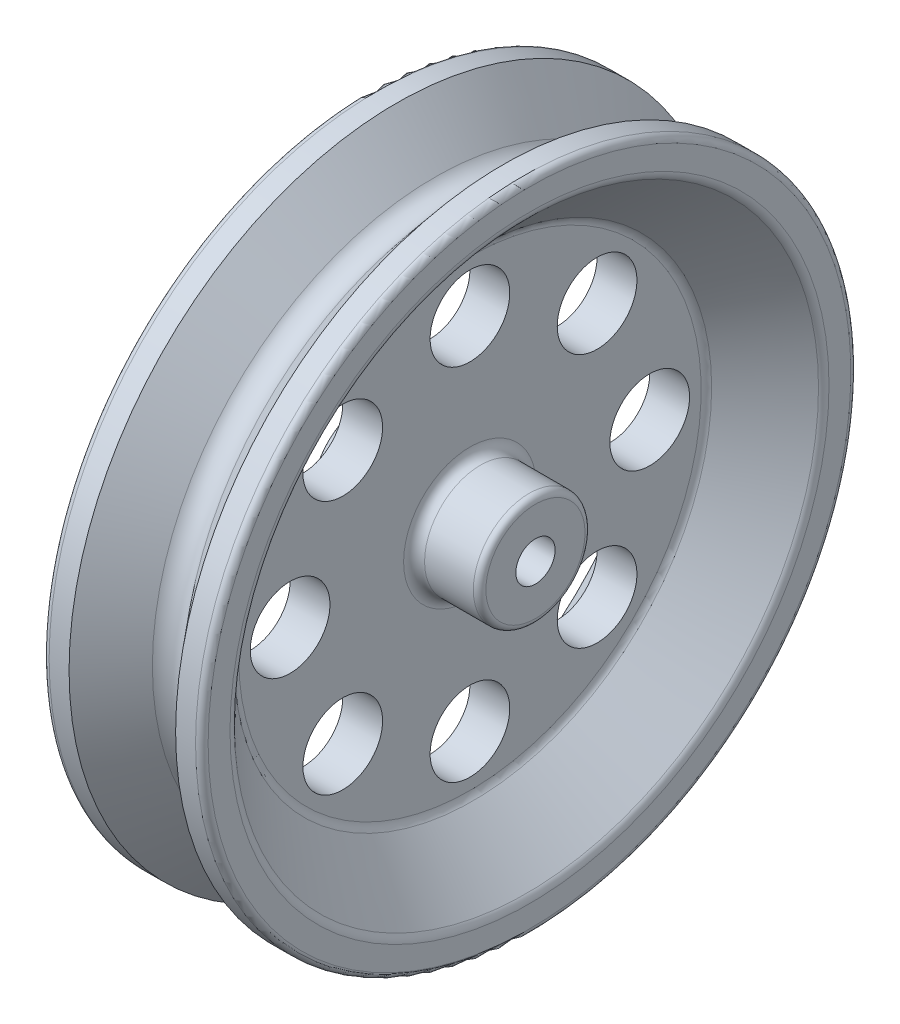
ISO-10303-21;
HEADER;
FILE_DESCRIPTION(('STEP AP214'),'2;1');
FILE_NAME('part.step','',(''),(''),'','','');
FILE_SCHEMA(('AUTOMOTIVE_DESIGN { 1 0 10303 214 1 1 1 1 }'));
ENDSEC;
DATA;
#1=APPLICATION_CONTEXT('core data for automotive mechanical design processes');
#2=APPLICATION_PROTOCOL_DEFINITION('international standard','automotive_design',2000,#1);
#3=PRODUCT_CONTEXT('',#1,'mechanical');
#4=PRODUCT('Part','Part','',(#3));
#5=PRODUCT_RELATED_PRODUCT_CATEGORY('part','',(#4));
#6=PRODUCT_DEFINITION_FORMATION('','',#4);
#7=PRODUCT_DEFINITION_CONTEXT('part definition',#1,'design');
#8=PRODUCT_DEFINITION('design','',#6,#7);
#9=PRODUCT_DEFINITION_SHAPE('','',#8);
#10=(LENGTH_UNIT() NAMED_UNIT(*) SI_UNIT(.MILLI.,.METRE.));
#11=(NAMED_UNIT(*) PLANE_ANGLE_UNIT() SI_UNIT($,.RADIAN.));
#12=(NAMED_UNIT(*) SI_UNIT($,.STERADIAN.) SOLID_ANGLE_UNIT());
#13=UNCERTAINTY_MEASURE_WITH_UNIT(LENGTH_MEASURE(1.E-05),#10,'distance_accuracy_value','');
#14=(GEOMETRIC_REPRESENTATION_CONTEXT(3) GLOBAL_UNCERTAINTY_ASSIGNED_CONTEXT((#13)) GLOBAL_UNIT_ASSIGNED_CONTEXT((#10,
#11,#12)) REPRESENTATION_CONTEXT('',''));
#15=CARTESIAN_POINT('',(0.,0.,0.));
#16=DIRECTION('',(0.,0.,1.));
#17=DIRECTION('',(1.,0.,0.));
#18=AXIS2_PLACEMENT_3D('',#15,#16,#17);
#19=CARTESIAN_POINT('',(0.,0.,0.));
#20=DIRECTION('',(-1.,0.,0.));
#21=DIRECTION('',(0.,0.,1.));
#22=AXIS2_PLACEMENT_3D('',#19,#20,#21);
#23=CYLINDRICAL_SURFACE('',#22,0.5325);
#24=CARTESIAN_POINT('',(-0.755,0.,0.));
#25=DIRECTION('',(1.,0.,0.));
#26=DIRECTION('',(0.,0.,-1.));
#27=AXIS2_PLACEMENT_3D('',#24,#25,#26);
#28=CIRCLE('',#27,0.5325);
#29=CARTESIAN_POINT('',(-0.755,0.,-0.5325));
#30=VERTEX_POINT('',#29);
#31=EDGE_CURVE('E10',#30,#30,#28,.T.);
#32=ORIENTED_EDGE('',*,*,#31,.T.);
#33=EDGE_LOOP('',(#32));
#34=FACE_BOUND('',#33,.T.);
#35=CARTESIAN_POINT('',(-0.29,0.,0.));
#36=DIRECTION('',(1.,0.,0.));
#37=DIRECTION('',(0.,0.,-1.));
#38=AXIS2_PLACEMENT_3D('',#35,#36,#37);
#39=CIRCLE('',#38,0.5325);
#40=CARTESIAN_POINT('',(-0.29,0.,-0.5325));
#41=VERTEX_POINT('',#40);
#42=EDGE_CURVE('E83',#41,#41,#39,.F.);
#43=ORIENTED_EDGE('',*,*,#42,.T.);
#44=EDGE_LOOP('',(#43));
#45=FACE_BOUND('',#44,.T.);
#46=ADVANCED_FACE('F40',(#34,#45),#23,.T.);
#47=CARTESIAN_POINT('',(-0.815,0.1875,0.));
#48=DIRECTION('',(1.,0.,0.));
#49=DIRECTION('',(0.,0.,-1.));
#50=AXIS2_PLACEMENT_3D('',#47,#48,#49);
#51=PLANE('',#50);
#52=CARTESIAN_POINT('',(-0.815,0.,0.));
#53=DIRECTION('',(1.,0.,0.));
#54=DIRECTION('',(0.,0.,-1.));
#55=AXIS2_PLACEMENT_3D('',#52,#53,#54);
#56=CIRCLE('',#55,0.4725);
#57=CARTESIAN_POINT('',(-0.815,0.,-0.4725));
#58=VERTEX_POINT('',#57);
#59=EDGE_CURVE('E42',#58,#58,#56,.F.);
#60=ORIENTED_EDGE('',*,*,#59,.T.);
#61=EDGE_LOOP('',(#60));
#62=FACE_BOUND('',#61,.T.);
#63=CARTESIAN_POINT('',(-0.815,0.,0.));
#64=DIRECTION('',(-1.,0.,0.));
#65=DIRECTION('',(0.,0.,1.));
#66=AXIS2_PLACEMENT_3D('',#63,#64,#65);
#67=CIRCLE('',#66,0.1875);
#68=CARTESIAN_POINT('',(-0.815,0.,0.1875));
#69=VERTEX_POINT('',#68);
#70=EDGE_CURVE('E104',#69,#69,#67,.T.);
#71=ORIENTED_EDGE('',*,*,#70,.F.);
#72=EDGE_LOOP('',(#71));
#73=FACE_BOUND('',#72,.T.);
#74=ADVANCED_FACE('F208',(#62,#73),#51,.F.);
#75=CARTESIAN_POINT('',(0.,0.,0.));
#76=DIRECTION('',(-1.,0.,0.));
#77=DIRECTION('',(0.,0.,1.));
#78=AXIS2_PLACEMENT_3D('',#75,#76,#77);
#79=CYLINDRICAL_SURFACE('',#78,0.1875);
#80=CARTESIAN_POINT('',(0.815,0.,0.));
#81=DIRECTION('',(-1.,0.,0.));
#82=DIRECTION('',(0.,0.,1.));
#83=AXIS2_PLACEMENT_3D('',#80,#81,#82);
#84=CIRCLE('',#83,0.1875);
#85=CARTESIAN_POINT('',(0.815,0.,0.1875));
#86=VERTEX_POINT('',#85);
#87=EDGE_CURVE('E107',#86,#86,#84,.T.);
#88=ORIENTED_EDGE('',*,*,#87,.F.);
#89=EDGE_LOOP('',(#88));
#90=FACE_BOUND('',#89,.T.);
#91=ORIENTED_EDGE('',*,*,#70,.T.);
#92=EDGE_LOOP('',(#91));
#93=FACE_BOUND('',#92,.T.);
#94=ADVANCED_FACE('F213',(#90,#93),#79,.F.);
#95=CARTESIAN_POINT('',(0.815,0.1875,0.));
#96=DIRECTION('',(-1.,0.,0.));
#97=DIRECTION('',(0.,0.,1.));
#98=AXIS2_PLACEMENT_3D('',#95,#96,#97);
#99=PLANE('',#98);
#100=CARTESIAN_POINT('',(0.815,0.,0.));
#101=DIRECTION('',(-1.,0.,0.));
#102=DIRECTION('',(0.,0.,1.));
#103=AXIS2_PLACEMENT_3D('',#100,#101,#102);
#104=CIRCLE('',#103,0.4725);
#105=CARTESIAN_POINT('',(0.815,0.,0.4725));
#106=VERTEX_POINT('',#105);
#107=EDGE_CURVE('E48',#106,#106,#104,.F.);
#108=ORIENTED_EDGE('',*,*,#107,.T.);
#109=EDGE_LOOP('',(#108));
#110=FACE_BOUND('',#109,.T.);
#111=ORIENTED_EDGE('',*,*,#87,.T.);
#112=EDGE_LOOP('',(#111));
#113=FACE_BOUND('',#112,.T.);
#114=ADVANCED_FACE('F282',(#110,#113),#99,.F.);
#115=CARTESIAN_POINT('',(0.,0.,0.));
#116=DIRECTION('',(-1.,0.,0.));
#117=DIRECTION('',(0.,0.,1.));
#118=AXIS2_PLACEMENT_3D('',#115,#116,#117);
#119=CYLINDRICAL_SURFACE('',#118,0.5325);
#120=CARTESIAN_POINT('',(0.755,0.,0.));
#121=DIRECTION('',(-1.,0.,0.));
#122=DIRECTION('',(0.,0.,1.));
#123=AXIS2_PLACEMENT_3D('',#120,#121,#122);
#124=CIRCLE('',#123,0.5325);
#125=CARTESIAN_POINT('',(0.755,0.,0.5325));
#126=VERTEX_POINT('',#125);
#127=EDGE_CURVE('E55',#126,#126,#124,.T.);
#128=ORIENTED_EDGE('',*,*,#127,.T.);
#129=EDGE_LOOP('',(#128));
#130=FACE_BOUND('',#129,.T.);
#131=CARTESIAN_POINT('',(0.29,0.,0.));
#132=DIRECTION('',(-1.,0.,0.));
#133=DIRECTION('',(0.,0.,1.));
#134=AXIS2_PLACEMENT_3D('',#131,#132,#133);
#135=CIRCLE('',#134,0.5325);
#136=CARTESIAN_POINT('',(0.29,0.,0.5325));
#137=VERTEX_POINT('',#136);
#138=EDGE_CURVE('E82',#137,#137,#135,.F.);
#139=ORIENTED_EDGE('',*,*,#138,.T.);
#140=EDGE_LOOP('',(#139));
#141=FACE_BOUND('',#140,.T.);
#142=ADVANCED_FACE('F283',(#130,#141),#119,.T.);
#143=CARTESIAN_POINT('',(0.19,0.5325,0.));
#144=DIRECTION('',(-1.,0.,0.));
#145=DIRECTION('',(0.,0.,1.));
#146=AXIS2_PLACEMENT_3D('',#143,#144,#145);
#147=PLANE('',#146);
#148=CARTESIAN_POINT('',(0.19,0.,-1.715));
#149=DIRECTION('',(-1.,0.,0.));
#150=DIRECTION('',(0.,0.,1.));
#151=AXIS2_PLACEMENT_3D('',#148,#149,#150);
#152=CIRCLE('',#151,0.38);
#153=CARTESIAN_POINT('',(0.19,0.,-1.335));
#154=VERTEX_POINT('',#153);
#155=EDGE_CURVE('E129',#154,#154,#152,.T.);
#156=ORIENTED_EDGE('',*,*,#155,.T.);
#157=EDGE_LOOP('',(#156));
#158=FACE_BOUND('',#157,.T.);
#159=CARTESIAN_POINT('',(0.19,-1.21268812973494,-1.21268812973492));
#160=DIRECTION('',(-1.,0.,0.));
#161=DIRECTION('',(0.,0.,1.));
#162=AXIS2_PLACEMENT_3D('',#159,#160,#161);
#163=CIRCLE('',#162,0.38);
#164=CARTESIAN_POINT('',(0.19,-1.21268812973494,-0.832688129734923));
#165=VERTEX_POINT('',#164);
#166=EDGE_CURVE('E135',#165,#165,#163,.T.);
#167=ORIENTED_EDGE('',*,*,#166,.T.);
#168=EDGE_LOOP('',(#167));
#169=FACE_BOUND('',#168,.T.);
#170=CARTESIAN_POINT('',(0.19,-1.715,0.));
#171=DIRECTION('',(-1.,0.,0.));
#172=DIRECTION('',(0.,0.,1.));
#173=AXIS2_PLACEMENT_3D('',#170,#171,#172);
#174=CIRCLE('',#173,0.38);
#175=CARTESIAN_POINT('',(0.19,-1.715,0.38));
#176=VERTEX_POINT('',#175);
#177=EDGE_CURVE('E132',#176,#176,#174,.T.);
#178=ORIENTED_EDGE('',*,*,#177,.T.);
#179=EDGE_LOOP('',(#178));
#180=FACE_BOUND('',#179,.T.);
#181=CARTESIAN_POINT('',(0.19,-1.21268812973492,1.21268812973494));
#182=DIRECTION('',(-1.,0.,0.));
#183=DIRECTION('',(0.,0.,1.));
#184=AXIS2_PLACEMENT_3D('',#181,#182,#183);
#185=CIRCLE('',#184,0.38);
#186=CARTESIAN_POINT('',(0.19,-1.21268812973492,1.59268812973494));
#187=VERTEX_POINT('',#186);
#188=EDGE_CURVE('E136',#187,#187,#185,.T.);
#189=ORIENTED_EDGE('',*,*,#188,.T.);
#190=EDGE_LOOP('',(#189));
#191=FACE_BOUND('',#190,.T.);
#192=CARTESIAN_POINT('',(0.19,0.,1.715));
#193=DIRECTION('',(-1.,0.,0.));
#194=DIRECTION('',(0.,0.,1.));
#195=AXIS2_PLACEMENT_3D('',#192,#193,#194);
#196=CIRCLE('',#195,0.38);
#197=CARTESIAN_POINT('',(0.19,0.,2.095));
#198=VERTEX_POINT('',#197);
#199=EDGE_CURVE('E143',#198,#198,#196,.T.);
#200=ORIENTED_EDGE('',*,*,#199,.T.);
#201=EDGE_LOOP('',(#200));
#202=FACE_BOUND('',#201,.T.);
#203=CARTESIAN_POINT('',(0.19,1.21268812973494,1.21268812973491));
#204=DIRECTION('',(-1.,0.,0.));
#205=DIRECTION('',(0.,0.,1.));
#206=AXIS2_PLACEMENT_3D('',#203,#204,#205);
#207=CIRCLE('',#206,0.38);
#208=CARTESIAN_POINT('',(0.19,1.21268812973494,1.59268812973491));
#209=VERTEX_POINT('',#208);
#210=EDGE_CURVE('E145',#209,#209,#207,.T.);
#211=ORIENTED_EDGE('',*,*,#210,.T.);
#212=EDGE_LOOP('',(#211));
#213=FACE_BOUND('',#212,.T.);
#214=CARTESIAN_POINT('',(0.19,1.21268812973493,-1.21268812973493));
#215=DIRECTION('',(-1.,0.,0.));
#216=DIRECTION('',(0.,0.,1.));
#217=AXIS2_PLACEMENT_3D('',#214,#215,#216);
#218=CIRCLE('',#217,0.38);
#219=CARTESIAN_POINT('',(0.19,1.21268812973493,-0.832688129734931));
#220=VERTEX_POINT('',#219);
#221=EDGE_CURVE('E150',#220,#220,#218,.T.);
#222=ORIENTED_EDGE('',*,*,#221,.T.);
#223=EDGE_LOOP('',(#222));
#224=FACE_BOUND('',#223,.T.);
#225=CARTESIAN_POINT('',(0.19,1.715,0.));
#226=DIRECTION('',(-1.,0.,0.));
#227=DIRECTION('',(0.,0.,1.));
#228=AXIS2_PLACEMENT_3D('',#225,#226,#227);
#229=CIRCLE('',#228,0.38);
#230=CARTESIAN_POINT('',(0.19,1.715,0.38));
#231=VERTEX_POINT('',#230);
#232=EDGE_CURVE('E121',#231,#231,#229,.T.);
#233=ORIENTED_EDGE('',*,*,#232,.T.);
#234=EDGE_LOOP('',(#233));
#235=FACE_BOUND('',#234,.T.);
#236=CARTESIAN_POINT('',(0.19,0.,0.));
#237=DIRECTION('',(-1.,0.,0.));
#238=DIRECTION('',(0.,0.,1.));
#239=AXIS2_PLACEMENT_3D('',#236,#237,#238);
#240=CIRCLE('',#239,0.6325);
#241=CARTESIAN_POINT('',(0.19,0.,0.6325));
#242=VERTEX_POINT('',#241);
#243=EDGE_CURVE('E87',#242,#242,#240,.T.);
#244=ORIENTED_EDGE('',*,*,#243,.T.);
#245=EDGE_LOOP('',(#244));
#246=FACE_BOUND('',#245,.T.);
#247=CARTESIAN_POINT('',(0.19,0.,0.));
#248=DIRECTION('',(-1.,0.,0.));
#249=DIRECTION('',(0.,0.,1.));
#250=AXIS2_PLACEMENT_3D('',#247,#248,#249);
#251=CIRCLE('',#250,2.20543037312372);
#252=CARTESIAN_POINT('',(0.19,0.,2.20543037312372));
#253=VERTEX_POINT('',#252);
#254=EDGE_CURVE('E89',#253,#253,#251,.F.);
#255=ORIENTED_EDGE('',*,*,#254,.T.);
#256=EDGE_LOOP('',(#255));
#257=FACE_BOUND('',#256,.T.);
#258=ADVANCED_FACE('F280',(#158,#169,#180,#191,#202,#213,#224,#235,#246,#257),#147,.F.);
#259=CARTESIAN_POINT('',(0.19,0.,0.));
#260=DIRECTION('',(1.,0.,0.));
#261=DIRECTION('',(0.,0.,-1.));
#262=AXIS2_PLACEMENT_3D('',#259,#260,#261);
#263=CONICAL_SURFACE('',#262,2.24685172936103,0.785398163397447);
#264=CARTESIAN_POINT('',(0.728858948756745,0.,0.));
#265=DIRECTION('',(-1.,0.,0.));
#266=DIRECTION('',(0.,0.,1.));
#267=AXIS2_PLACEMENT_3D('',#264,#265,#266);
#268=CIRCLE('',#267,2.78571067811777);
#269=CARTESIAN_POINT('',(0.728858948756745,0.,2.78571067811777));
#270=VERTEX_POINT('',#269);
#271=EDGE_CURVE('E60',#270,#270,#268,.F.);
#272=ORIENTED_EDGE('',*,*,#271,.T.);
#273=EDGE_LOOP('',(#272));
#274=FACE_BOUND('',#273,.T.);
#275=CARTESIAN_POINT('',(0.219289321881345,0.,0.));
#276=DIRECTION('',(1.,0.,0.));
#277=DIRECTION('',(0.,0.,-1.));
#278=AXIS2_PLACEMENT_3D('',#275,#276,#277);
#279=CIRCLE('',#278,2.27614105124237);
#280=CARTESIAN_POINT('',(0.219289321881345,0.,-2.27614105124237));
#281=VERTEX_POINT('',#280);
#282=EDGE_CURVE('E58',#281,#281,#279,.F.);
#283=ORIENTED_EDGE('',*,*,#282,.T.);
#284=EDGE_LOOP('',(#283));
#285=FACE_BOUND('',#284,.T.);
#286=ADVANCED_FACE('F247',(#274,#285),#263,.F.);
#287=CARTESIAN_POINT('',(0.75814827063809,2.81499999999912,0.));
#288=DIRECTION('',(-1.,0.,0.));
#289=DIRECTION('',(0.,0.,1.));
#290=AXIS2_PLACEMENT_3D('',#287,#288,#289);
#291=PLANE('',#290);
#292=CARTESIAN_POINT('',(0.75814827063809,0.,0.));
#293=DIRECTION('',(-1.,0.,0.));
#294=DIRECTION('',(0.,0.,1.));
#295=AXIS2_PLACEMENT_3D('',#292,#293,#294);
#296=CIRCLE('',#295,2.85642135623643);
#297=CARTESIAN_POINT('',(0.75814827063809,0.,2.85642135623643));
#298=VERTEX_POINT('',#297);
#299=EDGE_CURVE('E61',#298,#298,#296,.T.);
#300=ORIENTED_EDGE('',*,*,#299,.T.);
#301=EDGE_LOOP('',(#300));
#302=FACE_BOUND('',#301,.T.);
#303=CARTESIAN_POINT('',(0.75814827063809,0.,0.));
#304=DIRECTION('',(-1.,0.,0.));
#305=DIRECTION('',(0.,0.,1.));
#306=AXIS2_PLACEMENT_3D('',#303,#304,#305);
#307=CIRCLE('',#306,3.06499999999912);
#308=CARTESIAN_POINT('',(0.75814827063809,0.,3.06499999999912));
#309=VERTEX_POINT('',#308);
#310=EDGE_CURVE('E91',#309,#309,#307,.F.);
#311=ORIENTED_EDGE('',*,*,#310,.T.);
#312=EDGE_LOOP('',(#311));
#313=FACE_BOUND('',#312,.T.);
#314=ADVANCED_FACE('F242',(#302,#313),#291,.F.);
#315=CARTESIAN_POINT('',(0.,0.,0.));
#316=DIRECTION('',(-1.,0.,0.));
#317=DIRECTION('',(0.,0.,1.));
#318=AXIS2_PLACEMENT_3D('',#315,#316,#317);
#319=CYLINDRICAL_SURFACE('',#318,3.12499999999912);
#320=CARTESIAN_POINT('',(0.69814827063809,0.,0.));
#321=DIRECTION('',(-1.,0.,0.));
#322=DIRECTION('',(0.,0.,1.));
#323=AXIS2_PLACEMENT_3D('',#320,#321,#322);
#324=CIRCLE('',#323,3.12499999999912);
#325=CARTESIAN_POINT('',(0.69814827063809,0.,3.12499999999912));
#326=VERTEX_POINT('',#325);
#327=EDGE_CURVE('E96',#326,#326,#324,.T.);
#328=ORIENTED_EDGE('',*,*,#327,.T.);
#329=EDGE_LOOP('',(#328));
#330=FACE_BOUND('',#329,.T.);
#331=CARTESIAN_POINT('',(0.50814827063809,0.,0.));
#332=DIRECTION('',(-1.,0.,0.));
#333=DIRECTION('',(0.,0.,1.));
#334=AXIS2_PLACEMENT_3D('',#331,#332,#333);
#335=CIRCLE('',#334,3.12499999999912);
#336=CARTESIAN_POINT('',(0.50814827063809,0.,3.12499999999912));
#337=VERTEX_POINT('',#336);
#338=EDGE_CURVE('E112',#337,#337,#335,.T.);
#339=ORIENTED_EDGE('',*,*,#338,.F.);
#340=EDGE_LOOP('',(#339));
#341=FACE_BOUND('',#340,.T.);
#342=ADVANCED_FACE('F246',(#330,#341),#319,.T.);
#343=CARTESIAN_POINT('',(0.50814827063809,0.,0.));
#344=DIRECTION('',(1.,0.,0.));
#345=DIRECTION('',(0.,0.,-1.));
#346=AXIS2_PLACEMENT_3D('',#343,#344,#345);
#347=CONICAL_SURFACE('',#346,3.12499999999912,0.872664625997163);
#348=CARTESIAN_POINT('',(0.145548444192605,0.,0.));
#349=DIRECTION('',(-1.,0.,0.));
#350=DIRECTION('',(0.,0.,1.));
#351=AXIS2_PLACEMENT_3D('',#348,#349,#350);
#352=CIRCLE('',#351,2.69287035415868);
#353=CARTESIAN_POINT('',(0.145548444192605,0.,2.69287035415868));
#354=VERTEX_POINT('',#353);
#355=EDGE_CURVE('E111',#354,#354,#352,.T.);
#356=ORIENTED_EDGE('',*,*,#355,.F.);
#357=EDGE_LOOP('',(#356));
#358=FACE_BOUND('',#357,.T.);
#359=ORIENTED_EDGE('',*,*,#338,.T.);
#360=EDGE_LOOP('',(#359));
#361=FACE_BOUND('',#360,.T.);
#362=ADVANCED_FACE('F260',(#358,#361),#347,.T.);
#363=CARTESIAN_POINT('',(0.,0.,0.));
#364=DIRECTION('',(-1.,0.,0.));
#365=DIRECTION('',(0.,0.,1.));
#366=AXIS2_PLACEMENT_3D('',#363,#364,#365);
#367=TOROIDAL_SURFACE('',#366,2.81499999999912,0.19);
#368=CARTESIAN_POINT('',(-0.145548444192604,0.,0.));
#369=DIRECTION('',(-1.,0.,0.));
#370=DIRECTION('',(0.,0.,1.));
#371=AXIS2_PLACEMENT_3D('',#368,#369,#370);
#372=CIRCLE('',#371,2.69287035415867);
#373=CARTESIAN_POINT('',(-0.145548444192604,0.,2.69287035415867));
#374=VERTEX_POINT('',#373);
#375=EDGE_CURVE('E120',#374,#374,#372,.T.);
#376=ORIENTED_EDGE('',*,*,#375,.F.);
#377=EDGE_LOOP('',(#376));
#378=FACE_BOUND('',#377,.T.);
#379=ORIENTED_EDGE('',*,*,#355,.T.);
#380=EDGE_LOOP('',(#379));
#381=FACE_BOUND('',#380,.T.);
#382=ADVANCED_FACE('F265',(#378,#381),#367,.F.);
#383=CARTESIAN_POINT('',(-0.145548444192604,0.,0.));
#384=DIRECTION('',(-1.,0.,0.));
#385=DIRECTION('',(0.,0.,1.));
#386=AXIS2_PLACEMENT_3D('',#383,#384,#385);
#387=CONICAL_SURFACE('',#386,2.69287035415867,0.872664625997162);
#388=CARTESIAN_POINT('',(-0.50814827063809,0.,0.));
#389=DIRECTION('',(-1.,0.,0.));
#390=DIRECTION('',(0.,0.,1.));
#391=AXIS2_PLACEMENT_3D('',#388,#389,#390);
#392=CIRCLE('',#391,3.12499999999912);
#393=CARTESIAN_POINT('',(-0.50814827063809,0.,3.12499999999912));
#394=VERTEX_POINT('',#393);
#395=EDGE_CURVE('E117',#394,#394,#392,.T.);
#396=ORIENTED_EDGE('',*,*,#395,.F.);
#397=EDGE_LOOP('',(#396));
#398=FACE_BOUND('',#397,.T.);
#399=ORIENTED_EDGE('',*,*,#375,.T.);
#400=EDGE_LOOP('',(#399));
#401=FACE_BOUND('',#400,.T.);
#402=ADVANCED_FACE('F267',(#398,#401),#387,.T.);
#403=CARTESIAN_POINT('',(0.,0.,0.));
#404=DIRECTION('',(-1.,0.,0.));
#405=DIRECTION('',(0.,0.,1.));
#406=AXIS2_PLACEMENT_3D('',#403,#404,#405);
#407=CYLINDRICAL_SURFACE('',#406,3.12499999999912);
#408=CARTESIAN_POINT('',(-0.69814827063809,0.,0.));
#409=DIRECTION('',(1.,0.,0.));
#410=DIRECTION('',(0.,0.,-1.));
#411=AXIS2_PLACEMENT_3D('',#408,#409,#410);
#412=CIRCLE('',#411,3.12499999999912);
#413=CARTESIAN_POINT('',(-0.69814827063809,0.,-3.12499999999912));
#414=VERTEX_POINT('',#413);
#415=EDGE_CURVE('E97',#414,#414,#412,.T.);
#416=ORIENTED_EDGE('',*,*,#415,.T.);
#417=EDGE_LOOP('',(#416));
#418=FACE_BOUND('',#417,.T.);
#419=ORIENTED_EDGE('',*,*,#395,.T.);
#420=EDGE_LOOP('',(#419));
#421=FACE_BOUND('',#420,.T.);
#422=ADVANCED_FACE('F359',(#418,#421),#407,.T.);
#423=CARTESIAN_POINT('',(-0.75814827063809,2.81499999999912,0.));
#424=DIRECTION('',(1.,0.,0.));
#425=DIRECTION('',(0.,0.,-1.));
#426=AXIS2_PLACEMENT_3D('',#423,#424,#425);
#427=PLANE('',#426);
#428=CARTESIAN_POINT('',(-0.75814827063809,0.,0.));
#429=DIRECTION('',(1.,0.,0.));
#430=DIRECTION('',(0.,0.,-1.));
#431=AXIS2_PLACEMENT_3D('',#428,#429,#430);
#432=CIRCLE('',#431,2.85642135623643);
#433=CARTESIAN_POINT('',(-0.75814827063809,0.,-2.85642135623643));
#434=VERTEX_POINT('',#433);
#435=EDGE_CURVE('E68',#434,#434,#432,.T.);
#436=ORIENTED_EDGE('',*,*,#435,.T.);
#437=EDGE_LOOP('',(#436));
#438=FACE_BOUND('',#437,.T.);
#439=CARTESIAN_POINT('',(-0.75814827063809,0.,0.));
#440=DIRECTION('',(1.,0.,0.));
#441=DIRECTION('',(0.,0.,-1.));
#442=AXIS2_PLACEMENT_3D('',#439,#440,#441);
#443=CIRCLE('',#442,3.06499999999912);
#444=CARTESIAN_POINT('',(-0.75814827063809,0.,-3.06499999999912));
#445=VERTEX_POINT('',#444);
#446=EDGE_CURVE('E105',#445,#445,#443,.F.);
#447=ORIENTED_EDGE('',*,*,#446,.T.);
#448=EDGE_LOOP('',(#447));
#449=FACE_BOUND('',#448,.T.);
#450=ADVANCED_FACE('F366',(#438,#449),#427,.F.);
#451=CARTESIAN_POINT('',(-0.758148270638091,0.,0.));
#452=DIRECTION('',(-1.,0.,0.));
#453=DIRECTION('',(0.,0.,1.));
#454=AXIS2_PLACEMENT_3D('',#451,#452,#453);
#455=CONICAL_SURFACE('',#454,2.81499999999912,0.785398163397447);
#456=CARTESIAN_POINT('',(-0.728858948756745,0.,0.));
#457=DIRECTION('',(1.,0.,0.));
#458=DIRECTION('',(0.,0.,-1.));
#459=AXIS2_PLACEMENT_3D('',#456,#457,#458);
#460=CIRCLE('',#459,2.78571067811777);
#461=CARTESIAN_POINT('',(-0.728858948756745,0.,-2.78571067811777));
#462=VERTEX_POINT('',#461);
#463=EDGE_CURVE('E67',#462,#462,#460,.F.);
#464=ORIENTED_EDGE('',*,*,#463,.T.);
#465=EDGE_LOOP('',(#464));
#466=FACE_BOUND('',#465,.T.);
#467=CARTESIAN_POINT('',(-0.219289321881345,0.,0.));
#468=DIRECTION('',(-1.,0.,0.));
#469=DIRECTION('',(0.,0.,1.));
#470=AXIS2_PLACEMENT_3D('',#467,#468,#469);
#471=CIRCLE('',#470,2.27614105124237);
#472=CARTESIAN_POINT('',(-0.219289321881345,0.,2.27614105124237));
#473=VERTEX_POINT('',#472);
#474=EDGE_CURVE('E75',#473,#473,#471,.F.);
#475=ORIENTED_EDGE('',*,*,#474,.T.);
#476=EDGE_LOOP('',(#475));
#477=FACE_BOUND('',#476,.T.);
#478=ADVANCED_FACE('F177',(#466,#477),#455,.F.);
#479=CARTESIAN_POINT('',(-0.19,0.532499999999999,0.));
#480=DIRECTION('',(1.,0.,0.));
#481=DIRECTION('',(0.,0.,-1.));
#482=AXIS2_PLACEMENT_3D('',#479,#480,#481);
#483=PLANE('',#482);
#484=CARTESIAN_POINT('',(-0.19,0.,-1.715));
#485=DIRECTION('',(-1.,0.,0.));
#486=DIRECTION('',(0.,1.,0.));
#487=AXIS2_PLACEMENT_3D('',#484,#485,#486);
#488=CIRCLE('',#487,0.38);
#489=CARTESIAN_POINT('',(-0.19,0.379999999999994,-1.715));
#490=VERTEX_POINT('',#489);
#491=EDGE_CURVE('E153',#490,#490,#488,.T.);
#492=ORIENTED_EDGE('',*,*,#491,.F.);
#493=EDGE_LOOP('',(#492));
#494=FACE_BOUND('',#493,.T.);
#495=CARTESIAN_POINT('',(-0.19,-1.21268812973494,-1.21268812973492));
#496=DIRECTION('',(-1.,0.,0.));
#497=DIRECTION('',(0.,0.707106781186544,-0.707106781186551));
#498=AXIS2_PLACEMENT_3D('',#495,#496,#497);
#499=CIRCLE('',#498,0.38);
#500=CARTESIAN_POINT('',(-0.19,-0.943987552884049,-1.48138870658581));
#501=VERTEX_POINT('',#500);
#502=EDGE_CURVE('E161',#501,#501,#499,.T.);
#503=ORIENTED_EDGE('',*,*,#502,.F.);
#504=EDGE_LOOP('',(#503));
#505=FACE_BOUND('',#504,.T.);
#506=CARTESIAN_POINT('',(-0.19,-1.715,0.));
#507=DIRECTION('',(-1.,0.,0.));
#508=DIRECTION('',(0.,0.,-1.));
#509=AXIS2_PLACEMENT_3D('',#506,#507,#508);
#510=CIRCLE('',#509,0.38);
#511=CARTESIAN_POINT('',(-0.19,-1.715,-0.38));
#512=VERTEX_POINT('',#511);
#513=EDGE_CURVE('E160',#512,#512,#510,.T.);
#514=ORIENTED_EDGE('',*,*,#513,.F.);
#515=EDGE_LOOP('',(#514));
#516=FACE_BOUND('',#515,.T.);
#517=CARTESIAN_POINT('',(-0.19,-1.21268812973492,1.21268812973494));
#518=DIRECTION('',(-1.,0.,0.));
#519=DIRECTION('',(0.,-0.707106781186554,-0.707106781186541));
#520=AXIS2_PLACEMENT_3D('',#517,#518,#519);
#521=CIRCLE('',#520,0.38);
#522=CARTESIAN_POINT('',(-0.19,-1.48138870658581,0.943987552884054));
#523=VERTEX_POINT('',#522);
#524=EDGE_CURVE('E152',#523,#523,#521,.T.);
#525=ORIENTED_EDGE('',*,*,#524,.F.);
#526=EDGE_LOOP('',(#525));
#527=FACE_BOUND('',#526,.T.);
#528=CARTESIAN_POINT('',(-0.19,0.,1.715));
#529=DIRECTION('',(-1.,0.,0.));
#530=DIRECTION('',(0.,-1.,0.));
#531=AXIS2_PLACEMENT_3D('',#528,#529,#530);
#532=CIRCLE('',#531,0.38);
#533=CARTESIAN_POINT('',(-0.19,-0.379999999999982,1.715));
#534=VERTEX_POINT('',#533);
#535=EDGE_CURVE('E158',#534,#534,#532,.T.);
#536=ORIENTED_EDGE('',*,*,#535,.F.);
#537=EDGE_LOOP('',(#536));
#538=FACE_BOUND('',#537,.T.);
#539=CARTESIAN_POINT('',(-0.19,1.21268812973494,1.21268812973491));
#540=DIRECTION('',(-1.,0.,0.));
#541=DIRECTION('',(0.,-0.707106781186539,0.707106781186556));
#542=AXIS2_PLACEMENT_3D('',#539,#540,#541);
#543=CIRCLE('',#542,0.38);
#544=CARTESIAN_POINT('',(-0.19,0.943987552884059,1.48138870658581));
#545=VERTEX_POINT('',#544);
#546=EDGE_CURVE('E167',#545,#545,#543,.T.);
#547=ORIENTED_EDGE('',*,*,#546,.F.);
#548=EDGE_LOOP('',(#547));
#549=FACE_BOUND('',#548,.T.);
#550=CARTESIAN_POINT('',(-0.19,1.21268812973493,-1.21268812973493));
#551=DIRECTION('',(-1.,0.,0.));
#552=DIRECTION('',(0.,0.707106781186549,0.707106781186546));
#553=AXIS2_PLACEMENT_3D('',#550,#551,#552);
#554=CIRCLE('',#553,0.38);
#555=CARTESIAN_POINT('',(-0.19,1.48138870658582,-0.943987552884044));
#556=VERTEX_POINT('',#555);
#557=EDGE_CURVE('E147',#556,#556,#554,.T.);
#558=ORIENTED_EDGE('',*,*,#557,.F.);
#559=EDGE_LOOP('',(#558));
#560=FACE_BOUND('',#559,.T.);
#561=CARTESIAN_POINT('',(-0.19,1.715,0.));
#562=DIRECTION('',(-1.,0.,0.));
#563=DIRECTION('',(0.,0.,1.));
#564=AXIS2_PLACEMENT_3D('',#561,#562,#563);
#565=CIRCLE('',#564,0.38);
#566=CARTESIAN_POINT('',(-0.19,1.715,0.38));
#567=VERTEX_POINT('',#566);
#568=EDGE_CURVE('E127',#567,#567,#565,.T.);
#569=ORIENTED_EDGE('',*,*,#568,.F.);
#570=EDGE_LOOP('',(#569));
#571=FACE_BOUND('',#570,.T.);
#572=CARTESIAN_POINT('',(-0.19,0.,0.));
#573=DIRECTION('',(1.,0.,0.));
#574=DIRECTION('',(0.,0.,-1.));
#575=AXIS2_PLACEMENT_3D('',#572,#573,#574);
#576=CIRCLE('',#575,0.6325);
#577=CARTESIAN_POINT('',(-0.19,0.,-0.6325));
#578=VERTEX_POINT('',#577);
#579=EDGE_CURVE('E73',#578,#578,#576,.T.);
#580=ORIENTED_EDGE('',*,*,#579,.T.);
#581=EDGE_LOOP('',(#580));
#582=FACE_BOUND('',#581,.T.);
#583=CARTESIAN_POINT('',(-0.19,0.,0.));
#584=DIRECTION('',(1.,0.,0.));
#585=DIRECTION('',(0.,0.,-1.));
#586=AXIS2_PLACEMENT_3D('',#583,#584,#585);
#587=CIRCLE('',#586,2.20543037312372);
#588=CARTESIAN_POINT('',(-0.19,0.,-2.20543037312372));
#589=VERTEX_POINT('',#588);
#590=EDGE_CURVE('E76',#589,#589,#587,.F.);
#591=ORIENTED_EDGE('',*,*,#590,.T.);
#592=EDGE_LOOP('',(#591));
#593=FACE_BOUND('',#592,.T.);
#594=ADVANCED_FACE('F172',(#494,#505,#516,#527,#538,#549,#560,#571,#582,#593),#483,.F.);
#595=CARTESIAN_POINT('',(-0.69814827063809,0.,0.));
#596=DIRECTION('',(1.,0.,0.));
#597=DIRECTION('',(0.,0.,-1.));
#598=AXIS2_PLACEMENT_3D('',#595,#596,#597);
#599=TOROIDAL_SURFACE('',#598,3.06499999999912,0.06);
#600=ORIENTED_EDGE('',*,*,#415,.F.);
#601=EDGE_LOOP('',(#600));
#602=FACE_BOUND('',#601,.T.);
#603=ORIENTED_EDGE('',*,*,#446,.F.);
#604=EDGE_LOOP('',(#603));
#605=FACE_BOUND('',#604,.T.);
#606=ADVANCED_FACE('F176',(#602,#605),#599,.T.);
#607=CARTESIAN_POINT('',(0.69814827063809,0.,0.));
#608=DIRECTION('',(-1.,0.,0.));
#609=DIRECTION('',(0.,0.,1.));
#610=AXIS2_PLACEMENT_3D('',#607,#608,#609);
#611=TOROIDAL_SURFACE('',#610,3.06499999999912,0.06);
#612=ORIENTED_EDGE('',*,*,#310,.F.);
#613=EDGE_LOOP('',(#612));
#614=FACE_BOUND('',#613,.T.);
#615=ORIENTED_EDGE('',*,*,#327,.F.);
#616=EDGE_LOOP('',(#615));
#617=FACE_BOUND('',#616,.T.);
#618=ADVANCED_FACE('F219',(#614,#617),#611,.T.);
#619=CARTESIAN_POINT('',(0.29,0.,0.));
#620=DIRECTION('',(-1.,0.,0.));
#621=DIRECTION('',(0.,0.,1.));
#622=AXIS2_PLACEMENT_3D('',#619,#620,#621);
#623=TOROIDAL_SURFACE('',#622,0.6325,0.1);
#624=ORIENTED_EDGE('',*,*,#138,.F.);
#625=EDGE_LOOP('',(#624));
#626=FACE_BOUND('',#625,.T.);
#627=ORIENTED_EDGE('',*,*,#243,.F.);
#628=EDGE_LOOP('',(#627));
#629=FACE_BOUND('',#628,.T.);
#630=ADVANCED_FACE('F221',(#626,#629),#623,.F.);
#631=CARTESIAN_POINT('',(-0.29,0.,0.));
#632=DIRECTION('',(1.,0.,0.));
#633=DIRECTION('',(0.,0.,-1.));
#634=AXIS2_PLACEMENT_3D('',#631,#632,#633);
#635=TOROIDAL_SURFACE('',#634,0.6325,0.1);
#636=ORIENTED_EDGE('',*,*,#579,.F.);
#637=EDGE_LOOP('',(#636));
#638=FACE_BOUND('',#637,.T.);
#639=ORIENTED_EDGE('',*,*,#42,.F.);
#640=EDGE_LOOP('',(#639));
#641=FACE_BOUND('',#640,.T.);
#642=ADVANCED_FACE('F226',(#638,#641),#635,.F.);
#643=CARTESIAN_POINT('',(-0.65814827063809,0.,0.));
#644=DIRECTION('',(1.,0.,0.));
#645=DIRECTION('',(0.,0.,-1.));
#646=AXIS2_PLACEMENT_3D('',#643,#644,#645);
#647=TOROIDAL_SURFACE('',#646,2.85642135623643,0.1);
#648=ORIENTED_EDGE('',*,*,#435,.F.);
#649=EDGE_LOOP('',(#648));
#650=FACE_BOUND('',#649,.T.);
#651=ORIENTED_EDGE('',*,*,#463,.F.);
#652=EDGE_LOOP('',(#651));
#653=FACE_BOUND('',#652,.T.);
#654=ADVANCED_FACE('F235',(#650,#653),#647,.T.);
#655=CARTESIAN_POINT('',(0.65814827063809,0.,0.));
#656=DIRECTION('',(-1.,0.,0.));
#657=DIRECTION('',(0.,0.,1.));
#658=AXIS2_PLACEMENT_3D('',#655,#656,#657);
#659=TOROIDAL_SURFACE('',#658,2.85642135623643,0.1);
#660=ORIENTED_EDGE('',*,*,#271,.F.);
#661=EDGE_LOOP('',(#660));
#662=FACE_BOUND('',#661,.T.);
#663=ORIENTED_EDGE('',*,*,#299,.F.);
#664=EDGE_LOOP('',(#663));
#665=FACE_BOUND('',#664,.T.);
#666=ADVANCED_FACE('F204',(#662,#665),#659,.T.);
#667=CARTESIAN_POINT('',(0.29,0.,0.));
#668=DIRECTION('',(-1.,0.,0.));
#669=DIRECTION('',(0.,0.,1.));
#670=AXIS2_PLACEMENT_3D('',#667,#668,#669);
#671=TOROIDAL_SURFACE('',#670,2.20543037312372,0.1);
#672=ORIENTED_EDGE('',*,*,#254,.F.);
#673=EDGE_LOOP('',(#672));
#674=FACE_BOUND('',#673,.T.);
#675=ORIENTED_EDGE('',*,*,#282,.F.);
#676=EDGE_LOOP('',(#675));
#677=FACE_BOUND('',#676,.T.);
#678=ADVANCED_FACE('F194',(#674,#677),#671,.F.);
#679=CARTESIAN_POINT('',(-0.29,0.,0.));
#680=DIRECTION('',(1.,0.,0.));
#681=DIRECTION('',(0.,0.,-1.));
#682=AXIS2_PLACEMENT_3D('',#679,#680,#681);
#683=TOROIDAL_SURFACE('',#682,2.20543037312372,0.1);
#684=ORIENTED_EDGE('',*,*,#474,.F.);
#685=EDGE_LOOP('',(#684));
#686=FACE_BOUND('',#685,.T.);
#687=ORIENTED_EDGE('',*,*,#590,.F.);
#688=EDGE_LOOP('',(#687));
#689=FACE_BOUND('',#688,.T.);
#690=ADVANCED_FACE('F195',(#686,#689),#683,.F.);
#691=CARTESIAN_POINT('',(0.755,0.,0.));
#692=DIRECTION('',(-1.,0.,0.));
#693=DIRECTION('',(0.,0.,1.));
#694=AXIS2_PLACEMENT_3D('',#691,#692,#693);
#695=TOROIDAL_SURFACE('',#694,0.4725,0.06);
#696=ORIENTED_EDGE('',*,*,#107,.F.);
#697=EDGE_LOOP('',(#696));
#698=FACE_BOUND('',#697,.T.);
#699=ORIENTED_EDGE('',*,*,#127,.F.);
#700=EDGE_LOOP('',(#699));
#701=FACE_BOUND('',#700,.T.);
#702=ADVANCED_FACE('F192',(#698,#701),#695,.T.);
#703=CARTESIAN_POINT('',(-0.755,0.,0.));
#704=DIRECTION('',(1.,0.,0.));
#705=DIRECTION('',(0.,0.,-1.));
#706=AXIS2_PLACEMENT_3D('',#703,#704,#705);
#707=TOROIDAL_SURFACE('',#706,0.4725,0.06);
#708=ORIENTED_EDGE('',*,*,#31,.F.);
#709=EDGE_LOOP('',(#708));
#710=FACE_BOUND('',#709,.T.);
#711=ORIENTED_EDGE('',*,*,#59,.F.);
#712=EDGE_LOOP('',(#711));
#713=FACE_BOUND('',#712,.T.);
#714=ADVANCED_FACE('F39',(#710,#713),#707,.T.);
#715=CARTESIAN_POINT('',(0.815,1.715,0.));
#716=DIRECTION('',(-1.,0.,0.));
#717=DIRECTION('',(0.,0.,1.));
#718=AXIS2_PLACEMENT_3D('',#715,#716,#717);
#719=CYLINDRICAL_SURFACE('',#718,0.38);
#720=ORIENTED_EDGE('',*,*,#568,.T.);
#721=EDGE_LOOP('',(#720));
#722=FACE_BOUND('',#721,.T.);
#723=ORIENTED_EDGE('',*,*,#232,.F.);
#724=EDGE_LOOP('',(#723));
#725=FACE_BOUND('',#724,.T.);
#726=ADVANCED_FACE('F455',(#722,#725),#719,.F.);
#727=CARTESIAN_POINT('',(0.815,1.21268812973493,-1.21268812973493));
#728=DIRECTION('',(-1.,0.,0.));
#729=DIRECTION('',(0.,0.,1.));
#730=AXIS2_PLACEMENT_3D('',#727,#728,#729);
#731=CYLINDRICAL_SURFACE('',#730,0.38);
#732=ORIENTED_EDGE('',*,*,#557,.T.);
#733=EDGE_LOOP('',(#732));
#734=FACE_BOUND('',#733,.T.);
#735=ORIENTED_EDGE('',*,*,#221,.F.);
#736=EDGE_LOOP('',(#735));
#737=FACE_BOUND('',#736,.T.);
#738=ADVANCED_FACE('F458',(#734,#737),#731,.F.);
#739=CARTESIAN_POINT('',(0.815,1.21268812973494,1.21268812973491));
#740=DIRECTION('',(-1.,0.,0.));
#741=DIRECTION('',(0.,0.,1.));
#742=AXIS2_PLACEMENT_3D('',#739,#740,#741);
#743=CYLINDRICAL_SURFACE('',#742,0.38);
#744=ORIENTED_EDGE('',*,*,#546,.T.);
#745=EDGE_LOOP('',(#744));
#746=FACE_BOUND('',#745,.T.);
#747=ORIENTED_EDGE('',*,*,#210,.F.);
#748=EDGE_LOOP('',(#747));
#749=FACE_BOUND('',#748,.T.);
#750=ADVANCED_FACE('F467',(#746,#749),#743,.F.);
#751=CARTESIAN_POINT('',(0.815,0.,1.715));
#752=DIRECTION('',(-1.,0.,0.));
#753=DIRECTION('',(0.,0.,1.));
#754=AXIS2_PLACEMENT_3D('',#751,#752,#753);
#755=CYLINDRICAL_SURFACE('',#754,0.38);
#756=ORIENTED_EDGE('',*,*,#535,.T.);
#757=EDGE_LOOP('',(#756));
#758=FACE_BOUND('',#757,.T.);
#759=ORIENTED_EDGE('',*,*,#199,.F.);
#760=EDGE_LOOP('',(#759));
#761=FACE_BOUND('',#760,.T.);
#762=ADVANCED_FACE('F175',(#758,#761),#755,.F.);
#763=CARTESIAN_POINT('',(0.815,-1.21268812973492,1.21268812973494));
#764=DIRECTION('',(-1.,0.,0.));
#765=DIRECTION('',(0.,0.,1.));
#766=AXIS2_PLACEMENT_3D('',#763,#764,#765);
#767=CYLINDRICAL_SURFACE('',#766,0.38);
#768=ORIENTED_EDGE('',*,*,#524,.T.);
#769=EDGE_LOOP('',(#768));
#770=FACE_BOUND('',#769,.T.);
#771=ORIENTED_EDGE('',*,*,#188,.F.);
#772=EDGE_LOOP('',(#771));
#773=FACE_BOUND('',#772,.T.);
#774=ADVANCED_FACE('F488',(#770,#773),#767,.F.);
#775=CARTESIAN_POINT('',(0.815,-1.715,0.));
#776=DIRECTION('',(-1.,0.,0.));
#777=DIRECTION('',(0.,0.,1.));
#778=AXIS2_PLACEMENT_3D('',#775,#776,#777);
#779=CYLINDRICAL_SURFACE('',#778,0.38);
#780=ORIENTED_EDGE('',*,*,#513,.T.);
#781=EDGE_LOOP('',(#780));
#782=FACE_BOUND('',#781,.T.);
#783=ORIENTED_EDGE('',*,*,#177,.F.);
#784=EDGE_LOOP('',(#783));
#785=FACE_BOUND('',#784,.T.);
#786=ADVANCED_FACE('F500',(#782,#785),#779,.F.);
#787=CARTESIAN_POINT('',(0.815,-1.21268812973494,-1.21268812973492));
#788=DIRECTION('',(-1.,0.,0.));
#789=DIRECTION('',(0.,0.,1.));
#790=AXIS2_PLACEMENT_3D('',#787,#788,#789);
#791=CYLINDRICAL_SURFACE('',#790,0.38);
#792=ORIENTED_EDGE('',*,*,#502,.T.);
#793=EDGE_LOOP('',(#792));
#794=FACE_BOUND('',#793,.T.);
#795=ORIENTED_EDGE('',*,*,#166,.F.);
#796=EDGE_LOOP('',(#795));
#797=FACE_BOUND('',#796,.T.);
#798=ADVANCED_FACE('F510',(#794,#797),#791,.F.);
#799=CARTESIAN_POINT('',(0.815,0.,-1.715));
#800=DIRECTION('',(-1.,0.,0.));
#801=DIRECTION('',(0.,0.,1.));
#802=AXIS2_PLACEMENT_3D('',#799,#800,#801);
#803=CYLINDRICAL_SURFACE('',#802,0.38);
#804=ORIENTED_EDGE('',*,*,#491,.T.);
#805=EDGE_LOOP('',(#804));
#806=FACE_BOUND('',#805,.T.);
#807=ORIENTED_EDGE('',*,*,#155,.F.);
#808=EDGE_LOOP('',(#807));
#809=FACE_BOUND('',#808,.T.);
#810=ADVANCED_FACE('F520',(#806,#809),#803,.F.);
#811=CLOSED_SHELL('',(#46,#74,#94,#114,#142,#258,#286,#314,#342,#362,#382,#402,#422,#450,#478,
#594,#606,#618,#630,#642,#654,#666,#678,#690,#702,#714,#726,#738,#750,#762,#774,#786,#798,#810));
#812=MANIFOLD_SOLID_BREP('B2',#811);
#813=ADVANCED_BREP_SHAPE_REPRESENTATION('',(#18,#812),#14);
#814=SHAPE_DEFINITION_REPRESENTATION(#9,#813);
ENDSEC;
END-ISO-10303-21;
